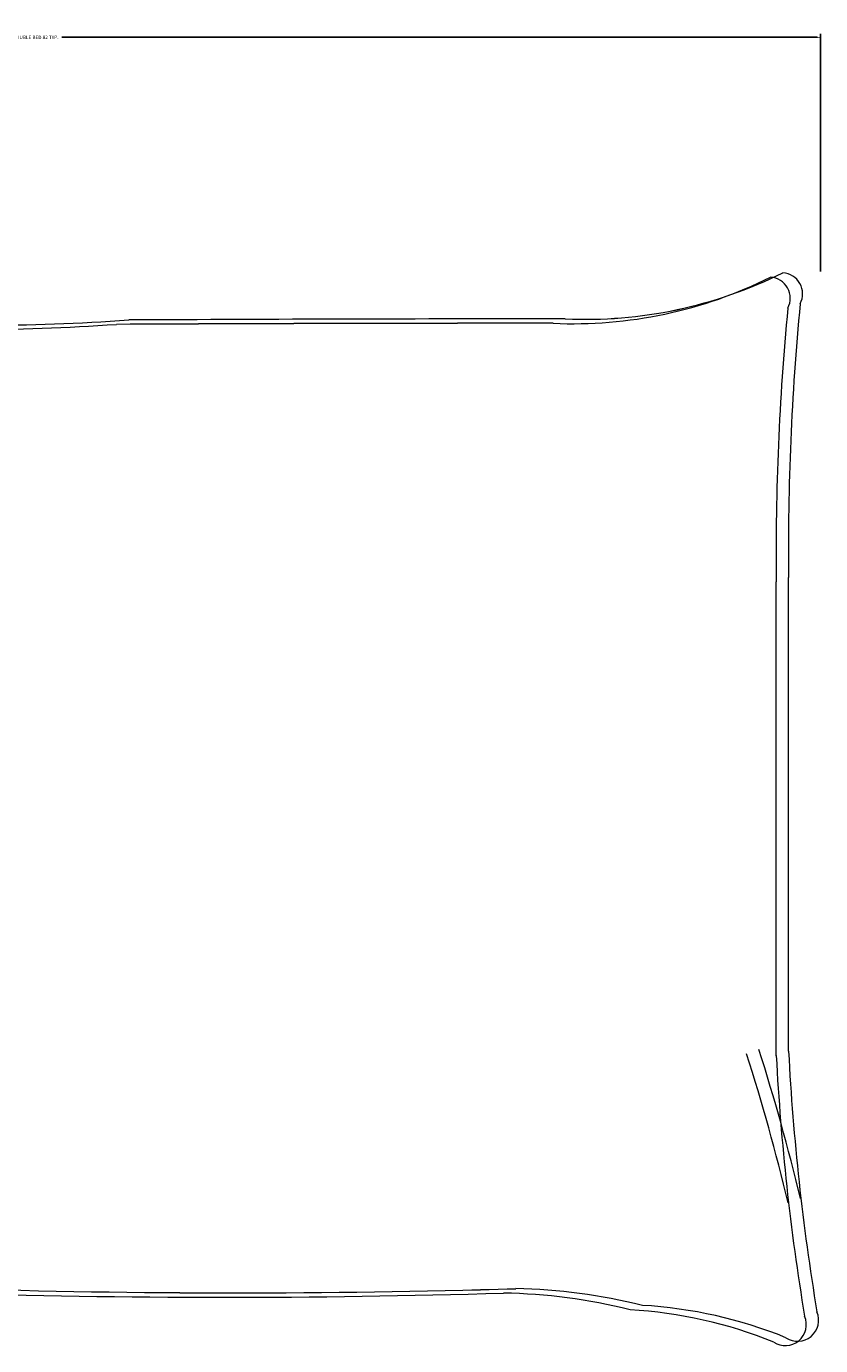
# Model space of a CAD drawing. Units: inches. Extents: x 963 to 2075, y 289 to 2657.
# Tile 42 of 98: x 1555 to 1597, y 1588 to 1656. Entities that reach past the tile are written whole.
import ezdxf

# ---------------------------------------------------------------- set-up
doc = ezdxf.new("R2010")
doc.units = ezdxf.units.IN
doc.layers.add('A-ANNO-DIMS', color=2, linetype='Continuous', lineweight=18)
doc.layers.add('A-FURN', color=8, linetype='Continuous', lineweight=18)
doc.styles.get("Standard").update_dxf_attribs({"font": 'arial.ttf'})
doc.dimstyles.get("Standard").update_dxf_attribs({"dimtxt": 0.18, "dimasz": 0.18, "dimexe": 0.18, "dimexo": 0.0625, "dimgap": 0.09, "dimtad": 0, "dimtih": 1, "dimtoh": 1, "dimdec": 4, "dimzin": 0, "dimdsep": 46, "dimtxsty": 'Standard', "dimcen": 0.09, "dimadec": 0, "dimazin": 0, "dimtfac": 1, "dimtdec": 4, "dimtofl": 0, "dimtmove": 0, "dimatfit": 3, "dimfxl": 1, "dimtolj": 1, "dimtzin": 0, "dimarcsym": 0})

# ---------------------------------------------------------------- blocks, each defined once
blk = doc.blocks.new('BED-DOUBLE')
for p, q in [((1174.987, 2438.932), (1174.987, 2414.318)), ((1174.987, 2438.931), (1174.987, 2414.317)), ((1175.627, 2439.16), (1175.627, 2414.546)), ((1175.627, 2439.16), (1175.627, 2414.546))]:
    blk.add_line(p, q)
for centre, radius, start, end in [((1174.515, 2452.907), 1.089, 56.17358, 203.47814), ((1174.515, 2452.907), 1.089, 56.17358, 203.47814), ((1175.154, 2453.136), 1.089, 56.17358, 203.47814), ((1175.154, 2453.135), 1.089, 56.17358, 203.47814), ((1183.957, 2475.654), 23.562, 247.97508, 266.652), ((1183.957, 2475.654), 23.562, 247.97508, 266.652), ((1184.596, 2475.882), 23.562, 247.97508, 266.652), ((1184.596, 2475.883), 23.562, 247.97508, 266.652), ((1053.395, 2432.568), 121.759, 2.99578, 9.40907), ((1053.395, 2432.568), 121.759, 2.99578, 9.40907), ((1054.035, 2432.796), 121.759, 2.99578, 9.40907), ((1054.035, 2432.796), 121.759, 2.99578, 9.40907), ((1189.717, 2480.894), 29.634, 256.06484, 268.91125), ((1189.717, 2480.894), 29.634, 256.06484, 268.91125), ((1190.357, 2481.123), 29.634, 256.06484, 268.91125), ((1190.357, 2481.123), 29.634, 256.06484, 268.91125), ((1203.619, 1969.172), 482.31, 88.22771, 91.71854), ((1203.619, 1969.173), 482.31, 88.22771, 91.71854), ((1204.258, 1969.401), 482.31, 88.22771, 91.71854), ((1204.258, 1969.401), 482.31, 88.22771, 91.71854), ((1277.944, 2471.216), 106.459, 193.38322, 197.70533), ((1277.944, 2471.217), 106.459, 193.38322, 197.70533), ((1278.584, 2471.445), 106.459, 193.38322, 197.70533), ((1278.584, 2471.445), 106.459, 193.38322, 197.70533), ((1041.956, 2412.843), 133.04, 354.4998, 0.63509), ((1041.956, 2412.843), 133.04, 354.4998, 0.63509), ((1042.595, 2413.071), 133.04, 354.4998, 0.63509), ((1042.595, 2413.071), 133.04, 354.4998, 0.63509), ((1186.205, 2378.066), 23.065, 87.47137, 116.46809), ((1186.205, 2378.066), 23.065, 87.47137, 116.46809), ((1187.05, 6962.966), 4561.858, 270.002168, 270.286888), ((1187.05, 6962.967), 4561.858, 270.002168, 270.286888), ((1217.917, 2271.729), 129.499, 86.97912, 93.83645), ((1217.917, 2271.729), 129.499, 86.97912, 93.83645), ((1218.557, 2271.957), 129.499, 86.97912, 93.83645), ((1218.557, 2271.957), 129.499, 86.97912, 93.83645), ((1176.002, 2399.813), 1.102, 152.65876, 266.02002), ((1176.002, 2399.813), 1.102, 152.65876, 266.02002), ((1185.566, 2377.837), 23.065, 87.47137, 116.46809), ((1185.566, 2377.838), 23.065, 87.47137, 116.46809), ((1186.411, 6962.738), 4561.858, 270.002168, 270.286888), ((1186.411, 6962.738), 4561.858, 270.002168, 270.286888), ((1175.362, 2399.585), 1.102, 152.65876, 266.02002), ((1175.362, 2399.585), 1.102, 152.65876, 266.02002)]:
    blk.add_arc(centre, radius, start, end)
blk = doc.blocks.new('*D14')
at = {"layer": 'A-ANNO-DIMS', "color": 0, "lineweight": -2, "transparency": 16777216}
for p, q in [((1515.065, 1643.568), (1515.065, 1655.918)), ((1515.245, 1655.738), (1554.47, 1655.738)), ((1596.434, 1655.738), (1557.208, 1655.738)), ((1596.614, 1643.568), (1596.614, 1655.918))]:
    blk.add_line(p, q, dxfattribs=at)
at = {"layer": 'A-ANNO-DIMS', "color": 0, "transparency": 16777216}
for points in [[(1515.245, 1655.768), (1515.245, 1655.708), (1515.065, 1655.738)], [(1596.434, 1655.768), (1596.434, 1655.708), (1596.614, 1655.738)]]:
    blk.add_solid(points, dxfattribs=at)
at = {"layer": 'Defpoints', "color": 0, "transparency": 16777216}
for p in [(1515.065, 1655.738), (1515.065, 1643.505), (1596.614, 1643.505)]:
    blk.add_point(p, dxfattribs=at)
at = {"layer": 'A-ANNO-DIMS', "color": 0, "transparency": 16777216, "insert": (1555.839, 1655.738), "char_height": 0.18, "attachment_point": 5}
blk.add_mtext('\\A1;DOUBLE BED 82 TYP.', dxfattribs=at)

msp = doc.modelspace()

# ---------------------------------------------------------------- block references
at = {"layer": 'A-FURN', "rotation": 180}
msp.add_blockref('BED-DOUBLE', (2769.937, 4041.99), dxfattribs=at)

# ---------------------------------------------------------------- dimensions: what is measured, and where the dimension line sits
at = {"layer": 'A-ANNO-DIMS'}
dim = msp.add_linear_dim(base=(1515.065, 1655.738), p1=(1596.614, 1643.505), p2=(1515.065, 1643.505), angle=180, text='DOUBLE BED <> TYP.', dimstyle='Standard', override={"dimdec": 0, "dimlfac": 1, "dimrnd": 0, "dimzin": 0, "dimdsep": 46, "dimlunit": 2}, dxfattribs=at)
dim.commit()
dim.dimension.update_dxf_attribs({"geometry": '*D14', "text_midpoint": (1555.839, 1655.738)})

doc.saveas('drawing.dxf')
